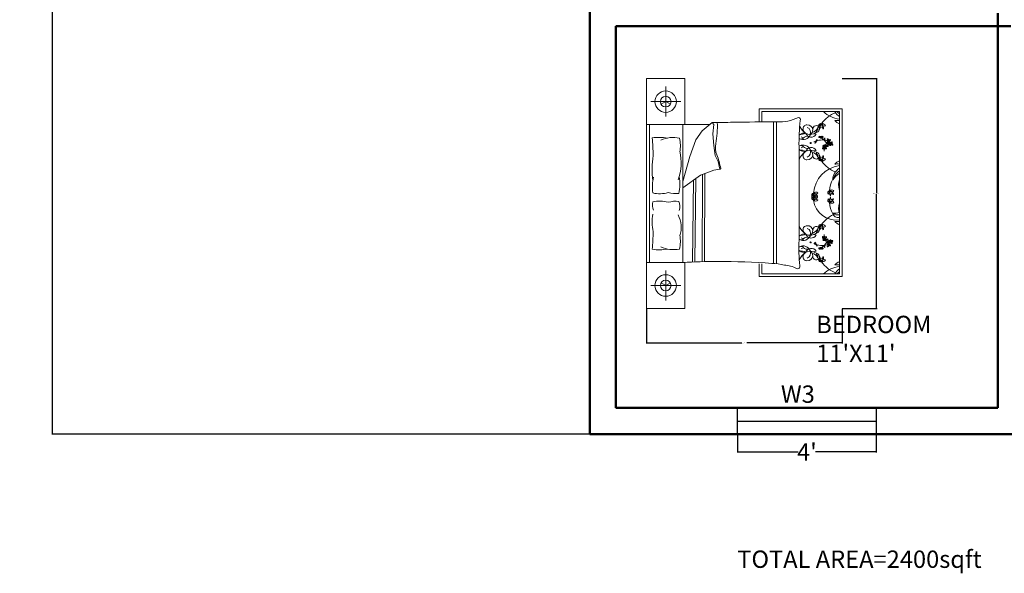
# Model space of a CAD drawing. Units: inches. Extents: x -173 to 545, y -746 to 104.
# Tile 1 of 32: x -173 to 168, y -746 to -554. Entities that reach past the tile are written whole.
import ezdxf

# ---------------------------------------------------------------- set-up
doc = ezdxf.new("R2010")
doc.units = ezdxf.units.IN
doc.header["$MEASUREMENT"] = 0
for name, color, linetype, lineweight in [('A-ANNO-DIMS', 2, 'Continuous', 18), ('A-ANNO-TEXT', 7, 'Continuous', 18), ('A-AREA-IDEN', 7, 'Continuous', 18), ('A-FURN', 8, 'Continuous', 18), ('A-GLAZ', 3, 'Continuous', 25), ('A-WALL', 7, 'Continuous', 50)]:
    doc.layers.add(name, color=color, linetype=linetype, lineweight=lineweight)
doc.styles.get("Standard").update_dxf_attribs({"font": 'arial.ttf'})
doc.dimstyles.get("Standard").update_dxf_attribs({"dimtxt": 0.18, "dimasz": 0.18, "dimexe": 0.18, "dimexo": 0.0625, "dimgap": 0.09, "dimtad": 0, "dimtih": 1, "dimtoh": 1, "dimdec": 0, "dimzin": 0, "dimdsep": 46, "dimlunit": 3, "dimtxsty": 'Standard', "dimcen": 0.09, "dimadec": 0, "dimazin": 0, "dimtfac": 1, "dimtdec": 0, "dimtofl": 0, "dimtmove": 0, "dimatfit": 3, "dimfxl": 1, "dimtolj": 1, "dimtzin": 0, "dimarcsym": 0})

# ---------------------------------------------------------------- blocks, each defined once
blk = doc.blocks.new('*D19')
at = {"layer": 'A-ANNO-DIMS', "color": 0, "lineweight": -2, "transparency": 16777216}
for p, q in [((75.3, -697.42), (75.3, -703.73)), ((123.3, -697.42), (123.3, -703.73)), ((75.48, -703.55), (96.33, -703.55)), ((123.12, -703.55), (102.27, -703.55))]:
    blk.add_line(p, q, dxfattribs=at)
at = {"layer": 'A-ANNO-DIMS', "color": 0, "transparency": 16777216}
for points in [[(75.48, -703.52), (75.48, -703.58), (75.3, -703.55)], [(123.12, -703.52), (123.12, -703.58), (123.3, -703.55)]]:
    blk.add_solid(points, dxfattribs=at)
at = {"layer": 'Defpoints', "color": 0, "transparency": 16777216}
for p in [(75.3, -697.36), (123.3, -697.36), (123.3, -703.55)]:
    blk.add_point(p, dxfattribs=at)
at = {"layer": 'A-ANNO-DIMS', "color": 0, "transparency": 16777216, "insert": (99.3, -703.55), "char_height": 6, "attachment_point": 5}
blk.add_mtext("\\A1;4'", dxfattribs=at)
blk = doc.blocks.new('*D24')
at = {"layer": 'A-ANNO-DIMS', "color": 0, "lineweight": -2, "transparency": 16777216}
for p, q in [((24.24, 16.64), (-161.72, 16.64)), ((-161.54, 16.46), (-161.54, -337.21)), ((-161.54, -697.18), (-161.54, -343.52)), ((24.24, -697.36), (-161.72, -697.36))]:
    blk.add_line(p, q, dxfattribs=at)
at = {"layer": 'A-ANNO-DIMS', "color": 0, "transparency": 16777216}
for points in [[(-161.57, 16.46), (-161.51, 16.46), (-161.54, 16.64)], [(-161.57, -697.18), (-161.51, -697.18), (-161.54, -697.36)]]:
    blk.add_solid(points, dxfattribs=at)
at = {"layer": 'Defpoints', "color": 0, "transparency": 16777216}
for p in [(24.3, 16.64), (-161.54, -697.36), (24.3, -697.36)]:
    blk.add_point(p, dxfattribs=at)
at = {"layer": 'A-ANNO-DIMS', "color": 0, "transparency": 16777216, "insert": (-161.54, -340.36), "char_height": 6, "attachment_point": 5}
blk.add_mtext('\\A1;59\'-6"', dxfattribs=at)
blk = doc.blocks.new('BED-SUITE-COMPACT')
for p, q in [((0, 79.47), (0, 0)), ((6.62, 66.33), (6.62, 76.71)), ((11.81, 71.52), (1.43, 71.52)), ((38.96, 68.98), (38.96, 64.48)), ((67.58, 68.98), (38.96, 68.98)), ((67.58, 11.04), (67.58, 68.98)), ((39.88, 64.49), (39.88, 68.06)), ((39.88, 68.06), (66.66, 68.06)), ((66.66, 68.06), (66.66, 11.96)), ((0, 63.58), (21.81, 63.58)), ((1.02, 15.89), (1.02, 63.58)), ((12.56, 63.58), (12.56, 15.89)), ((19.26, 61.39), (17.01, 58.33)), ((22.64, 64.29), (19.26, 61.39)), ((23.29, 63.64), (22.64, 64.29)), ((22.96, 60.42), (23.29, 63.64)), ((43.91, 15.53), (43.91, 64.49)), ((44.9, 15.46), (44.9, 64.49)), ((17.01, 58.33), (14.92, 52.54)), ((23.29, 56.4), (22.96, 60.42)), ((58.61, 60.23), (57.71, 60.4)), ((23.77, 52.86), (23.29, 56.4)), ((52.71, 23.6), (52.71, 55.87)), ((58.61, 54.67), (57.71, 54.5)), ((14.92, 52.54), (12.56, 43.87)), ((24.73, 50.77), (23.77, 52.86)), ((18.62, 46.1), (23.29, 47.87)), ((23.29, 47.87), (25.38, 48.19)), ((25.38, 48.19), (24.73, 50.77)), ((12.56, 41.74), (18.62, 46.1)), ((15.86, 16.11), (16.26, 44.4)), ((16.68, 16.14), (17.08, 44.99)), ((19.18, 16.18), (19.3, 46.36)), ((19.99, 16.17), (20.12, 46.67)), ((58.61, 25.35), (57.71, 25.53)), ((58.61, 19.8), (57.71, 19.62)), ((38.96, 15.45), (38.96, 11.04)), ((39.88, 11.96), (39.88, 15.47)), ((6.62, 13.14), (6.62, 2.75)), ((38.96, 11.04), (67.58, 11.04)), ((66.66, 11.96), (39.88, 11.96)), ((11.81, 7.95), (1.43, 7.95))]:
    blk.add_line(p, q)
for points in [[(13.24, 63.58), (13.24, 79.47), (0, 79.47)], [(6.62, 71.52), (5.02, 70.6)], [(6.62, 71.52), (8.23, 70.6)], [(0, 15.89), (13.24, 15.89), (13.24, 0), (0, 0)], [(6.62, 7.95), (5.02, 8.87)], [(6.62, 7.95), (8.23, 8.87)]]:
    blk.add_lwpolyline(points)
for points in [[(29.92, 64.45, -0.001242), (45, 64.49, 0.127202), (52.51, 66.08)], [(1.98, 59.01, -0.074897), (7.17, 58.91, 0.472817)], [(7.46, 40.11, -0.14099), (2.17, 39.95, -0.235245)], [(7.46, 36.71, 0.14099), (2.17, 36.87, 0.235245)], [(1.98, 20.46, 0.074897), (7.17, 20.55, -0.472817)], [(43.29, 15.55, -0.056112), (47.66, 14.98, -0.095341), (51.87, 13.86)]]:
    blk.add_lwpolyline(points, format="xyb")
for centre, radius in [((6.62, 71.52), 3.71), ((6.62, 71.52), 1.85), ((61.49, 55.64), 0.202), ((63.62, 56.96), 0.202), ((61.49, 24.39), 0.202), ((63.62, 23.06), 0.202), ((6.62, 7.95), 3.71), ((6.62, 7.95), 1.85)]:
    blk.add_circle(centre, radius)
for centre, radius, start, end in [((52.46, 65.35), 0.733, 332.6588, 86.02), ((135.43, 56.82), 82.73, 174.3113, 180.6567), ((69.09, 58.03), 10.38, 111.4092, 145.6135), ((68.06, 75.78), 10.38, 228.1144, 262.255), ((69.45, 70.58), 5.06, 209.8884, 236.5383), ((68.28, 67.75), 4.22, 221.0454, 247.4453), ((66.01, 79.3), 14.36, 266.3481, 272.5919), ((70.39, 72.4), 6.3, 223.5186, 233.6964), ((24.62, 137.15), 72.89, 268.447, 274.1706), ((-5.5, 62.93), 29.99, 348.6608, 2.5481), ((58.31, 65.66), 6.01, 206.7003, 236.3329), ((55.42, 62.16), 1.34, 88.9462, 185.5144), ((56.41, 62.57), 2.39, 193.079, 274.7067), ((55.61, 61.61), 1.9, 7.1143, 95.0551), ((54.89, 60.86), 1.84, 338.5779, 68.4181), ((55.19, 61.94), 2.31, 305.9599, 357.6409), ((56.04, 64.41), 3.75, 288.2955, 328.7386), ((58.67, 62.05), 1.19, 19.1312, 189.736), ((58.31, 62.33), 1.49, 285.6955, 4.031), ((60.29, 60.73), 1.59, 128.4175, 173.8338), ((59.96, 62.29), 0.731, 126.7319, 206.0245), ((60.32, 63.06), 0.86, 76.272, 177.0484), ((59.01, 64.81), 1.77, 284.7031, 328.6173), ((61.48, 62.56), 1.64, 125.7657, 194.5347), ((53.44, 65.47), 7.26, 332.8176, 347.4827), ((60.77, 62.77), 1.15, 20.9613, 102.2885), ((61.39, 63.92), 0.867, 181.7131, 301.5367), ((58.55, 62.16), 2.62, 2.0648, 41.1598), ((60.13, 63.14), 0.849, 316.2238, 62.3173), ((60.66, 62.63), 0.112, 20.2817, 316.2238), ((60.98, 62.27), 0.0626, 52.0591, 168.5166), ((61.04, 62.25), 0.129, 168.5166, 2.0648), ((-754.3, 15.21), 757.55, 2.85022, 3.31479), ((9.26, 48.89), 10.24, 78.2417, 114.8684), ((1.05, 56.18), 10.65, 348.9631, 14.8961), ((53.59, 59.38), 0.957, 206.442, 225.5483), ((53.59, 59.38), 0.957, 127.675, 149.9707), ((53.3, 63.46), 3.29, 260.8446, 301.1782), ((54.15, 60.91), 2.53, 240.8249, 340.7178), ((53.4, 59.78), 1.19, 246.1646, 318.4347), ((54.73, 57.6), 3.06, 85.2696, 124.215), ((54.61, 61.29), 2.28, 240.0851, 262.564), ((55.51, 57.91), 1.63, 74.8529, 138.4347), ((56.89, 61.21), 1.98, 196.8663, 330.0915), ((56.06, 59.96), 0.493, 254.8529, 12.6959), ((54.73, 57.6), 3.06, 53.6555, 57.2989), ((56.35, 64.45), 4.26, 273.4924, 303.7117), ((60.81, 51.71), 6.58, 110.1059, 116.9968), ((58.71, 57.9), 0.162, 112.5583, 214.2343), ((58.6, 58.19), 0.381, 265.7131, 351.6568), ((58.27, 58.4), 0.666, 297.3659, 329.344), ((57.77, 58.97), 1.28, 313.6929, 321.7899), ((59.18, 58.1), 0.417, 115.5379, 168.6744), ((57.76, 58.7), 1.26, 329.344, 349.7412), ((60.81, 51.71), 6.58, 86.1723, 106.4158), ((56.76, 58.41), 2.24, 352.8698, 1.6736), ((59.73, 59.22), 0.156, 125.0752, 284.7644), ((59.97, 59.28), 0.338, 127.3642, 168.4363), ((59.7, 59.55), 0.487, 277.4968, 341.2737), ((60.09, 59.32), 0.193, 88.1325, 178.8919), ((60.48, 59.12), 0.418, 136.3462, 189.6513), ((60.24, 59.08), 0.174, 189.6513, 312.3208), ((60.28, 59.56), 0.202, 183.2768, 356.7232), ((60.91, 59.2), 0.663, 164.2829, 186.9148), ((60.13, 59.19), 0.331, 312.3208, 40.2111), ((60.83, 59.57), 0.47, 201.6382, 274.947), ((60.21, 58.92), 0.614, 42.3896, 66.5724), ((66.41, 63.79), 7.55, 217.9541, 226.8459), ((60.66, 59.28), 0.334, 10.9597, 52.2379), ((60.86, 59.25), 0.155, 274.947, 37.5263), ((61.38, 58.37), 0.162, 112.5583, 214.2343), ((61.28, 58.66), 0.381, 265.7131, 351.6568), ((60.94, 58.87), 0.666, 297.3659, 329.344), ((60.98, 54.99), 3.3, 60.7959, 85.244), ((53.95, 50.24), 10.86, 37.8256, 47.7588), ((60.44, 59.45), 1.28, 313.6929, 321.7899), ((61.85, 58.57), 0.417, 115.5379, 168.6744), ((60.44, 59.17), 1.26, 329.344, 349.7412), ((59.43, 58.88), 2.24, 352.8698, 1.6736), ((62.58, 58.43), 0.226, 33.0979, 123.1364), ((57.61, 55.25), 5.91, 31.1156, 34.8118), ((62.26, 58.05), 0.612, 2.3172, 70.5201), ((62.76, 57.89), 0.177, 135.7354, 318.1297), ((62.47, 58.18), 0.234, 315.7354, 31.1156), ((62.89, 57.9), 0.177, 68.2452, 250.6395), ((62.49, 58.11), 0.527, 352.6008, 57.1845), ((62.99, 58.23), 0.527, 252.8042, 349.6943), ((63.05, 58.28), 0.234, 248.2452, 323.6254), ((62.84, 58.42), 0.612, 291.7087, 3.0299), ((58.47, 61.64), 5.91, 323.6254, 327.3216), ((63.32, 58.27), 0.226, 325.6077, 55.6462), ((30.25, 55.76), 6.47, 168.6608, 203.7384), ((53.59, 55.52), 0.957, 134.4517, 156.771), ((53.59, 55.52), 0.957, 203.2856, 232.325), ((53.3, 51.45), 3.29, 58.8218, 100.2867), ((54.15, 54), 2.53, 19.2822, 119.1751), ((53.4, 55.12), 1.19, 41.5653, 113.8354), ((54.73, 57.3), 3.06, 235.785, 274.7304), ((54.61, 53.61), 2.28, 97.436, 119.9149), ((56.41, 52.33), 2.39, 85.2933, 166.921), ((55.51, 56.99), 1.63, 221.5653, 285.1471), ((56.89, 53.69), 1.98, 29.9085, 163.1337), ((54.89, 54.04), 1.84, 291.5819, 21.4221), ((56.06, 54.94), 0.493, 347.3041, 105.1471), ((54.73, 57.3), 3.06, 302.7011, 306.3445), ((56.72, 57.24), 0.249, 169.5864, 349.5616), ((55.19, 52.96), 2.31, 2.3591, 54.0401), ((56.35, 50.46), 4.26, 56.2883, 86.5076), ((56.81, 57.22), 0.153, 349.5616, 167.2949), ((58.6, 57.14), 0.417, 129.5056, 182.6421), ((57.41, 58.1), 1.26, 308.4388, 328.836), ((57.19, 59.13), 2.24, 296.5064, 305.3102), ((57.17, 57.97), 1.28, 336.3901, 344.4871), ((58.56, 57.65), 0.162, 83.9457, 185.6216), ((57.91, 57.8), 0.666, 328.836, 0.8141), ((58.25, 57.6), 0.381, 306.5232, 32.4668), ((60.93, 55.3), 0.156, 125.0752, 284.7644), ((61.17, 55.36), 0.338, 93.635, 168.4363), ((61.18, 57.19), 0.923, 253.6301, 325.4631), ((61.44, 55.91), 0.653, 82.0748, 142.6895), ((61.37, 56.8), 0.67, 228.342, 274.9894), ((61.13, 55.89), 0.198, 138.2946, 276.2474), ((60.91, 55.63), 0.487, 277.4968, 341.2737), ((61.2, 55.86), 0.276, 358.5719, 143.8954), ((61.29, 55.4), 0.193, 88.1325, 178.8919), ((61.36, 56.08), 0.279, 208.8493, 269.9355), ((61.13, 56.01), 0.318, 274.2123, 318.1587), ((61.68, 55.2), 0.418, 136.3462, 189.6513), ((61.44, 55.15), 0.174, 189.6513, 312.3208), ((65.36, 54.65), 3.96, 175.2415, 182.8929), ((61.39, 56.69), 0.561, 273.8774, 357.1501), ((62.12, 55.27), 0.663, 164.2829, 186.9148), ((62.1, 55.69), 0.638, 121.9501, 165.2442), ((61.61, 57.09), 0.543, 262.0748, 308.2393), ((61.34, 55.27), 0.331, 312.3208, 40.2111), ((62.04, 55.64), 0.47, 201.6382, 274.947), ((61.66, 55.94), 0.134, 262.868, 7.094), ((61.41, 55), 0.614, 42.3896, 66.5724), ((61.64, 56.05), 0.399, 278.5614, 22.5914), ((61.86, 55.36), 0.334, 10.9597, 118.7804), ((65.36, 54.65), 3.96, 156.1523, 156.9499), ((61.87, 56.06), 0.201, 44.3732, 121.9501), ((62.48, 56.53), 0.561, 181.4625, 249.4747), ((62.39, 56.98), 0.543, 215.1128, 261.2773), ((62.82, 56.95), 0.923, 197.889, 269.722), ((65.36, 54.65), 3.96, 130.182, 149.456), ((62.06, 55.33), 0.155, 274.947, 37.5263), ((62.53, 56.63), 0.67, 248.3627, 295.0101), ((62.21, 55.79), 0.653, 20.6625, 81.2773), ((63.18, 56.91), 0.653, 139.3812, 199.9959), ((61.96, 57.38), 0.923, 310.9365, 22.7695), ((62.39, 57.33), 0.67, 285.6484, 332.2957), ((62.27, 57.69), 0.543, 319.3812, 5.5456), ((64.37, 54.58), 3.52, 111.7087, 116.2181), ((60.98, 54.99), 3.3, 47.5083, 55.9967), ((62.49, 57.29), 0.561, 331.1838, 51.6792), ((63.06, 56.62), 0.156, 125.0752, 284.7644), ((63.31, 56.68), 0.338, 93.635, 168.4363), ((63.26, 57.21), 0.198, 138.2946, 276.2474), ((63.04, 56.95), 0.487, 277.4968, 341.2737), ((63.34, 57.18), 0.276, 358.5719, 143.8954), ((63.43, 56.72), 0.193, 88.1325, 178.8919), ((63.5, 57.4), 0.279, 208.8493, 269.9355), ((63.26, 57.33), 0.318, 274.2123, 318.1587), ((63.82, 56.52), 0.418, 136.3462, 189.6513), ((63.58, 56.48), 0.174, 189.6513, 312.3208), ((64.25, 56.6), 0.663, 164.2829, 186.9148), ((64.23, 57.01), 0.638, 121.9501, 165.2442), ((63.47, 56.59), 0.331, 312.3208, 40.2111), ((64.17, 56.97), 0.47, 201.6382, 274.947), ((63.79, 57.26), 0.134, 262.868, 7.094), ((63.55, 56.32), 0.614, 42.3896, 66.5724), ((63.77, 57.37), 0.399, 278.5614, 22.5914), ((63.99, 56.68), 0.334, 10.9597, 118.7804), ((64, 57.39), 0.201, 44.3732, 121.9501), ((64.2, 56.65), 0.155, 274.947, 37.5263), ((30.74, 48.12), 28.82, 170.503, 187.7804), ((-6.52, 50.57), 18.47, 340.7385, 11.9603), ((-4.65, 42.67), 30.82, 10.6617, 19.8806), ((58.31, 49.24), 6.01, 123.6671, 158.5059), ((55.42, 52.74), 1.34, 174.4856, 271.0538), ((55.61, 53.29), 1.9, 264.9449, 352.8857), ((56.04, 50.49), 3.75, 31.2614, 71.7045), ((58.67, 52.86), 1.19, 170.264, 340.8688), ((60.29, 54.17), 1.59, 186.1662, 231.5825), ((58.31, 52.57), 1.49, 355.969, 74.3045), ((59.96, 52.61), 0.731, 153.9755, 233.2681), ((60.32, 51.85), 0.86, 182.9516, 283.728), ((59.01, 50.09), 1.77, 31.3827, 75.2969), ((61.48, 52.34), 1.64, 165.4653, 234.2343), ((53.44, 49.44), 7.26, 12.5173, 27.1824), ((58.55, 52.74), 2.62, 318.8402, 357.9352), ((60.13, 51.76), 0.849, 297.6827, 43.7762), ((61.39, 50.98), 0.867, 58.4633, 178.2869), ((60.77, 52.13), 1.15, 257.7115, 339.0387), ((60.62, 52.26), 0.0677, 43.7729, 339.7333), ((61.04, 52.65), 0.129, 357.9352, 191.4834), ((60.98, 52.63), 0.0626, 191.4834, 307.9409), ((25.44, 48.37), 0.192, 250.2464, 1.1377), ((68.06, 39.12), 10.38, 97.745, 175.5377), ((69.09, 56.87), 10.38, 214.3865, 248.5908), ((69.45, 44.32), 5.06, 123.4617, 178.728), ((68.28, 47.15), 4.22, 112.5547, 138.9546), ((66.01, 35.6), 14.36, 87.4081, 93.6519), ((16.17, 42.03), 14.16, 166.04, 188.4751), ((-2.49, 43.09), 14.01, 346.3762, 10.1383), ((73.62, 39.91), 10.38, 152.5854, 175.5377), ((70.39, 42.5), 6.3, 126.3036, 162.1496), ((72.17, 39.19), 9.37, 125.947, 145.9877), ((72.12, 42.81), 5.71, 162.9798, 196.4569), ((64.05, 39.87), 1.15, 50.8855, 132.2127), ((75.06, 40.55), 8.44, 174.3643, 175.6213), ((80.84, 36.11), 15.08, 160.0972, 160.2783), ((10.12, 49.47), 9.74, 254.1707, 275.9871), ((57.95, 39.1), 0.86, 106.1963, 206.9726), ((57.95, 38.28), 0.86, 153.0274, 253.8037), ((55.94, 39.97), 1.77, 314.6273, 358.5415), ((55.94, 37.41), 1.77, 1.4585, 45.3727), ((59.21, 39.25), 1.64, 155.6899, 224.4589), ((59.21, 38.13), 1.64, 135.5411, 204.3101), ((58.49, 39.07), 1.15, 50.8855, 132.2127), ((58.45, 40.38), 0.867, 211.6373, 331.4609), ((50.79, 37.75), 7.26, 2.7418, 17.407), ((57.75, 39.08), 0.849, 346.148, 92.2415), ((56.86, 37.44), 2.62, 31.989, 71.0841), ((50.79, 39.62), 7.26, 342.593, 357.2582), ((56.86, 39.93), 2.62, 288.9159, 328.011), ((57.75, 38.3), 0.849, 267.7585, 13.852), ((58.45, 37), 0.867, 28.5391, 148.3627), ((58.49, 38.3), 1.15, 227.7873, 309.1145), ((65.66, 38.59), 8.03, 188.1803, 277.1364), ((58.46, 38.9), 0.112, 50.0755, 346.148), ((58.42, 38.49), 0.0677, 13.9791, 309.8091), ((58.98, 38.76), 0.129, 198.4408, 31.989), ((58.92, 38.74), 0.0626, 81.9833, 198.4408), ((58.98, 38.61), 0.129, 328.011, 161.5592), ((58.92, 38.63), 0.0626, 161.5592, 278.0167), ((63.51, 39.89), 0.86, 106.1963, 206.9726), ((63.51, 37.48), 0.86, 153.0274, 253.8037), ((61.5, 40.76), 1.77, 314.6273, 358.5415), ((61.5, 36.61), 1.77, 1.4585, 45.3727), ((64.77, 40.04), 1.64, 155.6899, 224.4589), ((64.77, 37.33), 1.64, 135.5411, 204.3101), ((64.01, 41.17), 0.867, 211.6373, 331.4609), ((62.42, 38.24), 2.62, 31.989, 71.0841), ((56.35, 38.55), 7.26, 2.7418, 17.407), ((63.31, 39.87), 0.849, 346.148, 92.2415), ((56.35, 38.83), 7.26, 342.593, 357.2582), ((62.42, 39.14), 2.62, 288.9159, 328.011), ((63.31, 37.5), 0.849, 267.7585, 13.852), ((64.02, 39.69), 0.112, 50.0755, 346.148), ((63.98, 37.69), 0.0677, 13.9791, 309.8091), ((64.48, 39.54), 0.0626, 81.9833, 198.4408), ((64.48, 37.84), 0.0626, 161.5592, 278.0167), ((64.54, 39.56), 0.129, 198.4408, 31.989), ((64.54, 37.82), 0.129, 328.011, 161.5592), ((5.94, 35.78), 3.93, 163.8974, 206.6563), ((10.12, 27.35), 9.74, 84.0129, 105.8293), ((7.31, 35.25), 4.21, 341.4593, 24.9817), ((64.01, 36.2), 0.867, 28.5391, 148.3627), ((64.05, 37.51), 1.15, 227.7873, 309.1145), ((73.62, 37.46), 10.38, 184.4623, 207.4146), ((72.12, 34.56), 5.71, 163.5431, 197.0202), ((75.06, 36.82), 8.44, 184.3787, 185.6357), ((80.84, 41.27), 15.08, 199.7217, 199.9028), ((15.89, 29.89), 13.97, 168.8159, 193.6573), ((1.84, 27.89), 10.12, 343.8254, 26.1239), ((69.09, 23.15), 10.38, 111.4092, 145.6135), ((64.93, 37.55), 4.65, 263.3805, 291.883), ((66.22, 33.29), 1.86, 190.9261, 283.6102), ((65.97, 34.69), 2.36, 228.0951, 287.1391), ((58.31, 30.78), 6.01, 201.4941, 236.3329), ((55.42, 27.28), 1.34, 88.9462, 185.5144), ((55.61, 26.73), 1.9, 7.1143, 95.0551), ((54.89, 25.98), 1.84, 338.5779, 68.4181), ((56.04, 29.53), 3.75, 288.2955, 328.7386), ((58.67, 27.17), 1.19, 19.1312, 189.736), ((58.31, 27.45), 1.49, 285.6955, 4.031), ((59.96, 27.41), 0.731, 126.7319, 206.0245), ((60.32, 28.18), 0.86, 76.272, 177.0484), ((59.01, 29.94), 1.77, 284.7031, 328.6173), ((61.48, 27.68), 1.64, 125.7657, 194.5347), ((53.44, 30.59), 7.26, 332.8176, 347.4827), ((60.77, 27.89), 1.15, 20.9613, 102.2885), ((60.13, 28.26), 0.849, 316.2238, 62.3173), ((58.55, 27.29), 2.62, 2.0648, 41.1598), ((61.39, 29.04), 0.867, 181.7131, 301.5367), ((60.66, 27.75), 0.112, 20.2817, 316.2238), ((60.98, 27.39), 0.0626, 52.0591, 168.5166), ((61.04, 27.38), 0.129, 168.5166, 2.0648), ((66.01, 44.43), 14.36, 266.3481, 272.5919), ((68.28, 32.87), 4.22, 221.0454, 247.4453), ((-754.3, 64.26), 757.55, 356.68521, 357.14978), ((1.05, 23.29), 10.65, 345.1039, 11.0369), ((53.3, 28.58), 3.29, 259.7133, 301.1782), ((53.59, 24.5), 0.957, 127.675, 156.7144), ((53.59, 24.5), 0.957, 203.2856, 225.5483), ((54.15, 26.03), 2.53, 240.8249, 340.7178), ((53.4, 24.9), 1.19, 246.1646, 318.4347), ((54.73, 22.72), 3.06, 85.2696, 124.215), ((54.61, 26.41), 2.28, 240.0851, 262.564), ((56.41, 27.69), 2.39, 193.079, 274.7067), ((55.51, 23.04), 1.63, 74.8529, 138.4347), ((56.89, 26.33), 1.98, 196.8663, 330.0915), ((56.06, 25.08), 0.493, 254.8529, 12.6959), ((54.73, 22.72), 3.06, 53.6555, 57.2989), ((55.19, 27.06), 2.31, 305.9599, 357.6409), ((56.35, 29.57), 4.26, 273.4924, 303.7117), ((60.29, 25.85), 1.59, 128.4175, 173.8338), ((60.93, 24.73), 0.156, 75.2356, 234.9248), ((61.17, 24.67), 0.338, 191.5637, 266.365), ((61.37, 23.22), 0.67, 85.0106, 131.658), ((61.13, 24.13), 0.198, 83.7526, 221.7054), ((60.91, 24.4), 0.487, 18.7263, 82.5032), ((61.2, 24.16), 0.276, 216.1046, 1.4281), ((61.29, 24.62), 0.193, 181.1081, 271.8675), ((61.36, 23.95), 0.279, 90.0645, 151.1507), ((61.13, 24.01), 0.318, 41.8413, 85.7877), ((61.68, 24.83), 0.418, 170.3487, 223.6538), ((61.44, 24.87), 0.174, 47.6792, 170.3487), ((65.36, 25.37), 3.96, 177.1071, 184.7585), ((61.39, 23.33), 0.561, 2.8499, 86.1226), ((62.12, 24.75), 0.663, 173.0852, 195.7171), ((62.1, 24.33), 0.638, 194.7558, 238.0499), ((61.34, 24.75), 0.331, 319.7889, 47.6792), ((62.04, 24.38), 0.47, 85.053, 158.3618), ((61.66, 24.09), 0.134, 352.906, 97.132), ((61.41, 25.02), 0.614, 293.4276, 317.6104), ((61.86, 24.66), 0.334, 241.2196, 349.0403), ((61.64, 23.97), 0.399, 337.4086, 81.4386), ((62.48, 23.49), 0.561, 110.5253, 178.5375), ((62.82, 23.08), 0.923, 90.278, 162.111), ((62.06, 24.69), 0.155, 322.4737, 85.053), ((62.53, 23.39), 0.67, 64.9899, 111.6373), ((62.21, 24.23), 0.653, 278.7227, 339.3375), ((9.26, 30.58), 10.24, 245.1316, 281.7583), ((130, 21.17), 77.33, 178.1965, 184.7598), ((53.59, 20.64), 0.957, 134.4517, 163.3657), ((54.15, 19.12), 2.53, 19.2822, 119.1751), ((53.4, 20.24), 1.19, 41.5653, 113.8354), ((54.61, 18.73), 2.28, 97.436, 119.9149), ((55.51, 22.11), 1.63, 221.5653, 285.1471), ((56.89, 18.81), 1.98, 29.9085, 163.1337), ((56.06, 20.06), 0.493, 347.3041, 105.1471), ((56.72, 22.78), 0.249, 10.4384, 190.4136), ((56.81, 22.8), 0.153, 192.7051, 10.4384), ((60.81, 28.31), 6.58, 243.0032, 249.8941), ((57.41, 21.92), 1.26, 31.164, 51.5612), ((58.6, 22.88), 0.417, 177.3579, 230.4944), ((57.19, 20.9), 2.24, 54.6898, 63.4936), ((57.17, 22.05), 1.28, 15.5129, 23.6099), ((58.56, 22.38), 0.162, 174.3784, 276.0543), ((58.25, 22.42), 0.381, 327.5332, 53.4768), ((57.91, 22.22), 0.666, 359.1859, 31.164), ((58.71, 22.12), 0.162, 145.7657, 247.4417), ((58.6, 21.83), 0.381, 8.3432, 94.2869), ((58.27, 21.62), 0.666, 30.656, 62.6341), ((57.77, 21.05), 1.28, 38.2101, 46.3071), ((59.18, 21.92), 0.417, 191.3256, 244.4621), ((57.76, 21.32), 1.26, 10.2588, 30.656), ((60.81, 28.31), 6.58, 253.5842, 273.8277), ((56.76, 21.61), 2.24, 358.3264, 7.1302), ((59.73, 20.8), 0.156, 75.2356, 234.9248), ((59.97, 20.74), 0.338, 191.5637, 232.6358), ((59.7, 20.47), 0.487, 18.7263, 82.5032), ((60.09, 20.7), 0.193, 181.1081, 271.8675), ((60.48, 20.9), 0.418, 170.3487, 223.6538), ((60.24, 20.95), 0.174, 47.6792, 170.3487), ((60.28, 20.46), 0.202, 3.2768, 176.7232), ((60.91, 20.83), 0.663, 173.0852, 195.7171), ((60.13, 20.83), 0.331, 319.7889, 47.6792), ((60.83, 20.46), 0.47, 85.053, 158.3618), ((66.41, 16.24), 7.55, 133.1541, 142.0459), ((60.21, 21.1), 0.614, 293.4276, 317.6104), ((60.66, 20.74), 0.334, 307.7621, 349.0403), ((60.86, 20.77), 0.155, 322.4737, 85.053), ((61.18, 22.84), 0.923, 34.5369, 106.3699), ((61.44, 24.12), 0.653, 217.3105, 277.9252), ((61.38, 21.65), 0.162, 145.7657, 247.4417), ((53.95, 29.78), 10.86, 312.2412, 322.1744), ((60.98, 25.03), 3.3, 274.756, 299.2041), ((61.28, 21.36), 0.381, 8.3432, 94.2869), ((60.94, 21.15), 0.666, 30.656, 62.6341), ((60.44, 20.58), 1.28, 38.2101, 46.3071), ((61.85, 21.45), 0.417, 191.3256, 244.4621), ((60.44, 20.85), 1.26, 10.2588, 30.656), ((61.61, 22.93), 0.543, 51.7607, 97.9252), ((59.43, 21.14), 2.24, 358.3264, 7.1302), ((65.36, 25.37), 3.96, 203.0501, 203.8477), ((61.87, 23.96), 0.201, 238.0499, 315.6268), ((62.39, 23.05), 0.543, 98.7227, 144.8872), ((65.36, 25.37), 3.96, 210.544, 229.818), ((62.26, 21.98), 0.612, 289.4799, 357.6828), ((57.61, 24.78), 5.91, 325.1882, 328.8844), ((62.58, 21.59), 0.226, 236.8636, 326.9021), ((63.18, 23.12), 0.653, 160.0041, 220.6188), ((61.96, 22.64), 0.923, 337.2305, 49.0635), ((62.39, 22.69), 0.67, 27.7043, 74.3516), ((62.76, 22.13), 0.177, 41.8703, 224.2646), ((62.47, 21.84), 0.234, 328.8844, 44.2646), ((62.27, 22.34), 0.543, 354.4544, 40.6188), ((62.89, 22.13), 0.177, 109.3605, 291.7548), ((62.49, 21.91), 0.527, 302.8155, 7.3992), ((64.37, 25.45), 3.52, 243.7819, 248.2913), ((60.98, 25.03), 3.3, 304.0033, 312.4917), ((62.49, 22.73), 0.561, 308.3208, 28.8162), ((62.99, 21.79), 0.527, 10.3057, 107.1958), ((63.06, 23.4), 0.156, 75.2356, 234.9248), ((63.05, 21.75), 0.234, 36.3746, 111.7548), ((63.31, 23.34), 0.338, 191.5637, 266.365), ((63.26, 22.81), 0.198, 83.7526, 221.7054), ((62.84, 21.6), 0.612, 356.9701, 68.2913), ((63.04, 23.07), 0.487, 18.7263, 82.5032), ((63.34, 22.84), 0.276, 216.1046, 1.4281), ((63.43, 23.3), 0.193, 181.1081, 271.8675), ((58.47, 18.38), 5.91, 32.6784, 36.3746), ((63.5, 22.62), 0.279, 90.0645, 151.1507), ((63.26, 22.69), 0.318, 41.8413, 85.7877), ((63.58, 23.55), 0.174, 47.6792, 170.3487), ((63.82, 23.5), 0.418, 170.3487, 223.6538), ((63.32, 21.76), 0.226, 304.3538, 34.3923), ((64.25, 23.42), 0.663, 173.0852, 195.7171), ((64.23, 23.01), 0.638, 194.7558, 238.0499), ((63.47, 23.43), 0.331, 319.7889, 47.6792), ((64.17, 23.06), 0.47, 85.053, 158.3618), ((63.79, 22.76), 0.134, 352.906, 97.132), ((63.55, 23.7), 0.614, 293.4276, 317.6104), ((63.99, 23.34), 0.334, 241.2196, 349.0403), ((63.77, 22.65), 0.399, 337.4086, 81.4386), ((64, 22.64), 0.201, 238.0499, 315.6268), ((64.2, 23.37), 0.155, 322.4737, 85.053), ((53.59, 20.64), 0.957, 197.4186, 232.325), ((53.3, 16.57), 3.29, 58.8218, 100.751), ((58.31, 14.36), 6.01, 123.6671, 156.3547), ((54.73, 22.42), 3.06, 235.785, 274.7304), ((56.41, 17.45), 2.39, 85.2933, 166.921), ((55.42, 17.86), 1.34, 174.4856, 271.0538), ((55.61, 18.41), 1.9, 264.9449, 352.8857), ((54.89, 19.16), 1.84, 291.5819, 21.4221), ((54.73, 22.42), 3.06, 302.7011, 306.3445), ((55.19, 18.08), 2.31, 2.3591, 54.0401), ((56.35, 15.58), 4.26, 56.2883, 86.5076), ((56.04, 15.61), 3.75, 31.2614, 71.7045), ((58.67, 17.98), 1.19, 170.264, 340.8688), ((58.31, 17.69), 1.49, 355.969, 74.3045), ((60.29, 19.3), 1.59, 186.1662, 231.5825), ((59.96, 17.73), 0.731, 153.9755, 233.2681), ((61.48, 17.46), 1.64, 165.4653, 234.2343), ((53.44, 14.56), 7.26, 12.5173, 27.1824), ((58.55, 17.86), 2.62, 318.8402, 357.9352), ((60.13, 16.88), 0.849, 297.6827, 43.7762), ((60.62, 17.38), 0.0677, 43.7729, 339.7333), ((61.04, 17.77), 0.129, 357.9352, 191.4834), ((60.98, 17.76), 0.0626, 191.4834, 307.9409), ((22.27, -126.57), 142.79, 89.0718, 93.9), ((27.46, -170.04), 186.27, 85.1265, 90.8855), ((52.27, 14.46), 0.724, 236.1736, 23.4781), ((59.01, 15.21), 1.77, 31.3827, 75.2969), ((60.32, 16.97), 0.86, 182.9516, 283.728), ((61.39, 16.11), 0.867, 58.4633, 178.2869), ((60.77, 17.26), 1.15, 257.7115, 339.0387), ((69.09, 21.99), 10.38, 214.3865, 248.5908), ((68.06, 4.24), 10.38, 97.745, 131.8856), ((69.45, 9.44), 5.06, 123.4617, 150.1116), ((68.28, 12.28), 4.22, 112.5547, 138.9546), ((66.01, 0.72), 14.36, 87.4081, 93.6519), ((70.39, 7.63), 6.3, 126.3036, 136.4814)]:
    blk.add_arc(centre, radius, start, end)
blk = doc.blocks.new('WINDOW-48')
for p, q in [((0, 9), (48, 9)), ((0, 0), (0, 9)), ((48, 9), (48, 0)), ((0, 4.5), (48, 4.5)), ((48, 0), (0, 0))]:
    blk.add_line(p, q)
blk = doc.blocks.new('*D62')
at = {"layer": 'A-ANNO-DIMS', "color": 0, "lineweight": -2, "transparency": 16777216}
for p, q in [((111.52, -574.49), (123.56, -574.49)), ((123.38, -574.67), (123.38, -614.04)), ((123.38, -653.78), (123.38, -614.41)), ((111.52, -653.96), (123.56, -653.96))]:
    blk.add_line(p, q, dxfattribs=at)
at = {"layer": 'A-ANNO-DIMS', "color": 0, "transparency": 16777216}
for points in [[(123.35, -574.67), (123.41, -574.67), (123.38, -574.49)], [(123.35, -653.78), (123.41, -653.78), (123.38, -653.96)]]:
    blk.add_solid(points, dxfattribs=at)
at = {"layer": 'Defpoints', "color": 0, "transparency": 16777216}
for p in [(111.46, -574.49), (123.38, -574.49), (111.46, -653.96)]:
    blk.add_point(p, dxfattribs=at)
at = {"layer": 'A-ANNO-DIMS', "color": 0, "transparency": 16777216, "insert": (123.38, -614.23), "char_height": 0.18, "attachment_point": 5}
blk.add_mtext('\\A1;BED SET 6\'-7 1/2" TYP.', dxfattribs=at)
blk = doc.blocks.new('*D63')
at = {"layer": 'A-ANNO-DIMS', "color": 0, "lineweight": -2, "transparency": 16777216}
for p, q in [((43.87, -654.02), (43.87, -666.06)), ((111.46, -654.02), (111.46, -666.06)), ((44.05, -665.88), (76.82, -665.88)), ((111.28, -665.88), (78.51, -665.88))]:
    blk.add_line(p, q, dxfattribs=at)
at = {"layer": 'A-ANNO-DIMS', "color": 0, "transparency": 16777216}
for points in [[(44.05, -665.85), (44.05, -665.91), (43.87, -665.88)], [(111.28, -665.85), (111.28, -665.91), (111.46, -665.88)]]:
    blk.add_solid(points, dxfattribs=at)
at = {"layer": 'Defpoints', "color": 0, "transparency": 16777216}
for p in [(43.87, -653.96), (111.46, -653.96), (111.46, -665.88)]:
    blk.add_point(p, dxfattribs=at)
at = {"layer": 'A-ANNO-DIMS', "color": 0, "transparency": 16777216, "insert": (77.67, -665.88), "char_height": 0.18, "attachment_point": 5}
blk.add_mtext('\\A1;5\'-7 1/2" TYP.', dxfattribs=at)

msp = doc.modelspace()

# ---------------------------------------------------------------- linework, layer by layer
at = {"layer": 'A-WALL'}
for p, q in [((24.3, 16.64), (24.3, -697.36)), ((165.3, -551.86), (165.3, -688.36)), ((33.3, -556.36), (169.8, -556.36)), ((33.3, -556.36), (33.3, -688.36)), ((33.3, -688.36), (165.3, -688.36)), ((24.3, -697.36), (501.8, -697.36))]:
    msp.add_line(p, q, dxfattribs=at)

# ---------------------------------------------------------------- block references
at = {"layer": 'A-FURN'}
msp.add_blockref('BED-SUITE-COMPACT', (43.87, -653.96), dxfattribs=at)
at = {"layer": 'A-GLAZ'}
msp.add_blockref('WINDOW-48', (75.3, -697.36), dxfattribs=at)

# ---------------------------------------------------------------- texts
at = {"layer": 'A-ANNO-TEXT', "insert": (90.31, -680.57), "char_height": 6, "attachment_point": 1}
msp.add_mtext('W3', dxfattribs=at)
at = {"layer": 'A-AREA-IDEN', "char_height": 6, "attachment_point": 1}
for s, insert in [("BEDROOM\\P11'X11'", (102.53, -656.48)), ('TOTAL AREA=2400sqft', (75.23, -737.64))]:
    msp.add_mtext(s, dxfattribs=dict(at, insert=insert))

# ---------------------------------------------------------------- dimensions: what is measured, and where the dimension line sits
at = {"layer": 'A-ANNO-DIMS'}
dim = msp.add_linear_dim(base=(-161.54, -697.36), p1=(24.3, 16.64), p2=(24.3, -697.36), angle=90, dimstyle='Standard', override={"dimtxt": 6, "dimclrd": 0, "dimclre": 0, "dimclrt": 0}, dxfattribs=at)
dim.commit()
dim.dimension.update_dxf_attribs({"geometry": '*D24', "text_midpoint": (-161.54, -340.36)})
dim = msp.add_linear_dim(base=(123.38, -574.49), p1=(111.46, -653.96), p2=(111.46, -574.49), angle=90, text='BED SET <> TYP.', dimstyle='Standard', override={"dimdec": 1, "dimlfac": 1, "dimrnd": 0, "dimzin": 1, "dimdsep": 46, "dimlunit": 4, "dimfrac": 2}, dxfattribs=at)
dim.commit()
dim.dimension.update_dxf_attribs({"geometry": '*D62', "text_midpoint": (123.38, -614.23)})
dim = msp.add_linear_dim(base=(111.46, -665.88), p1=(43.87, -653.96), p2=(111.46, -653.96), text='<> TYP.', dimstyle='Standard', override={"dimdec": 1, "dimlfac": 1, "dimrnd": 0, "dimzin": 1, "dimdsep": 46, "dimlunit": 4, "dimfrac": 2}, dxfattribs=at)
dim.commit()
dim.dimension.update_dxf_attribs({"geometry": '*D63', "text_midpoint": (77.67, -665.88)})
dim = msp.add_linear_dim(base=(123.3, -703.55), p1=(75.3, -697.36), p2=(123.3, -697.36), dimstyle='Standard', override={"dimtxt": 6, "dimclrd": 0, "dimclre": 0, "dimclrt": 0}, dxfattribs=at)
dim.commit()
dim.dimension.update_dxf_attribs({"geometry": '*D19', "text_midpoint": (99.3, -703.55)})

doc.saveas('drawing.dxf')
